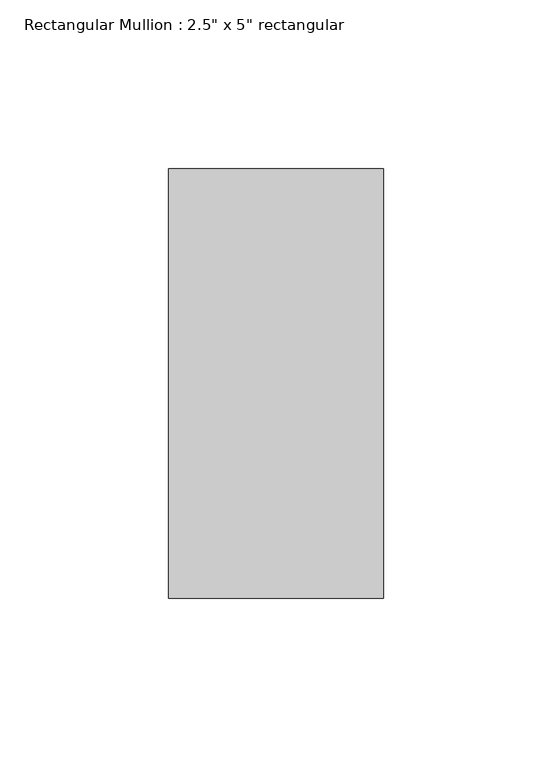
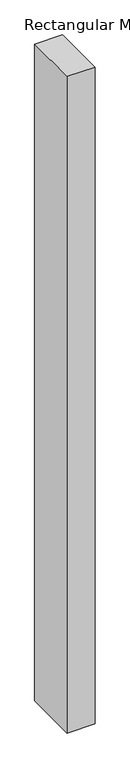
"""IFC4 building model written with IfcOpenShell, lengths in millimetres: member geometry."""

from ifc_helpers import new_model, si_unit, frame, origin, place, context, project, spatial, polyline, outline, extrude, source, transform, mapped, element, save


def member_d9ff3611(model_context):
    return source(origin(), model_context, "Body", "SweptSolid", [
        extrude(outline(polyline([(31.75, 63.5), (31.75, -63.5), (-31.75, -63.5), (-31.75, 63.5), (31.75, 63.5)])), frame((0.0, 0.0, -1574.1253432), z_axis=(0.0, 0.0, 1.0), x_axis=(1.0, 0.0, 0.0)), (0.0, 0.0, 1.0), 1574.1253432),
    ])


if __name__ == "__main__":
    model = new_model("IFC4")
    model_context = context("Model", 3, world=origin())
    ifc_project = project(units=[si_unit("LENGTHUNIT", "METRE", prefix="MILLI")], contexts=[model_context])
    site = spatial("IfcSite", under=ifc_project)
    building = spatial("IfcBuilding", under=site)
    placement = place(None, origin())
    member_shape = member_d9ff3611(model_context)
    element("IfcMember", 1, ObjectType="Rectangular Mullion : 2.5\" x 5\" rectangular", at=placement, inside=building, context=model_context, shape_type="MappedRepresentation", body=[
        mapped(member_shape, transform((0.0, 0.0, 0.0), x_axis=(1.0, 0.0, 0.0), y_axis=(0.0, 1.0, 0.0), z_axis=(0.0, 0.0, 1.0))),
    ])
    save(model, "model.ifc")

# Revit data of these elements
# Type "Rectangular Mullion : 2.5\" x 5\" rectangular"
#   built-in parameter 1007304 = 0.416667 (stored number, unit not read)
#   built-in parameter 1007301 = 0.104167 (stored number, unit not read)
#   built-in parameter 1007300 = 0.104167 (stored number, unit not read)
# Element 1 (IfcMember, "Rectangular Mullion : 2.5\" x 5\" rectangular")
#   Materials on its faces: "Aluminum"
# Materials
#   "Aluminum": class "Metal", colour RGB 247 247 247, transparency 0, Description = "Aluminum 6061", Cost = 0
